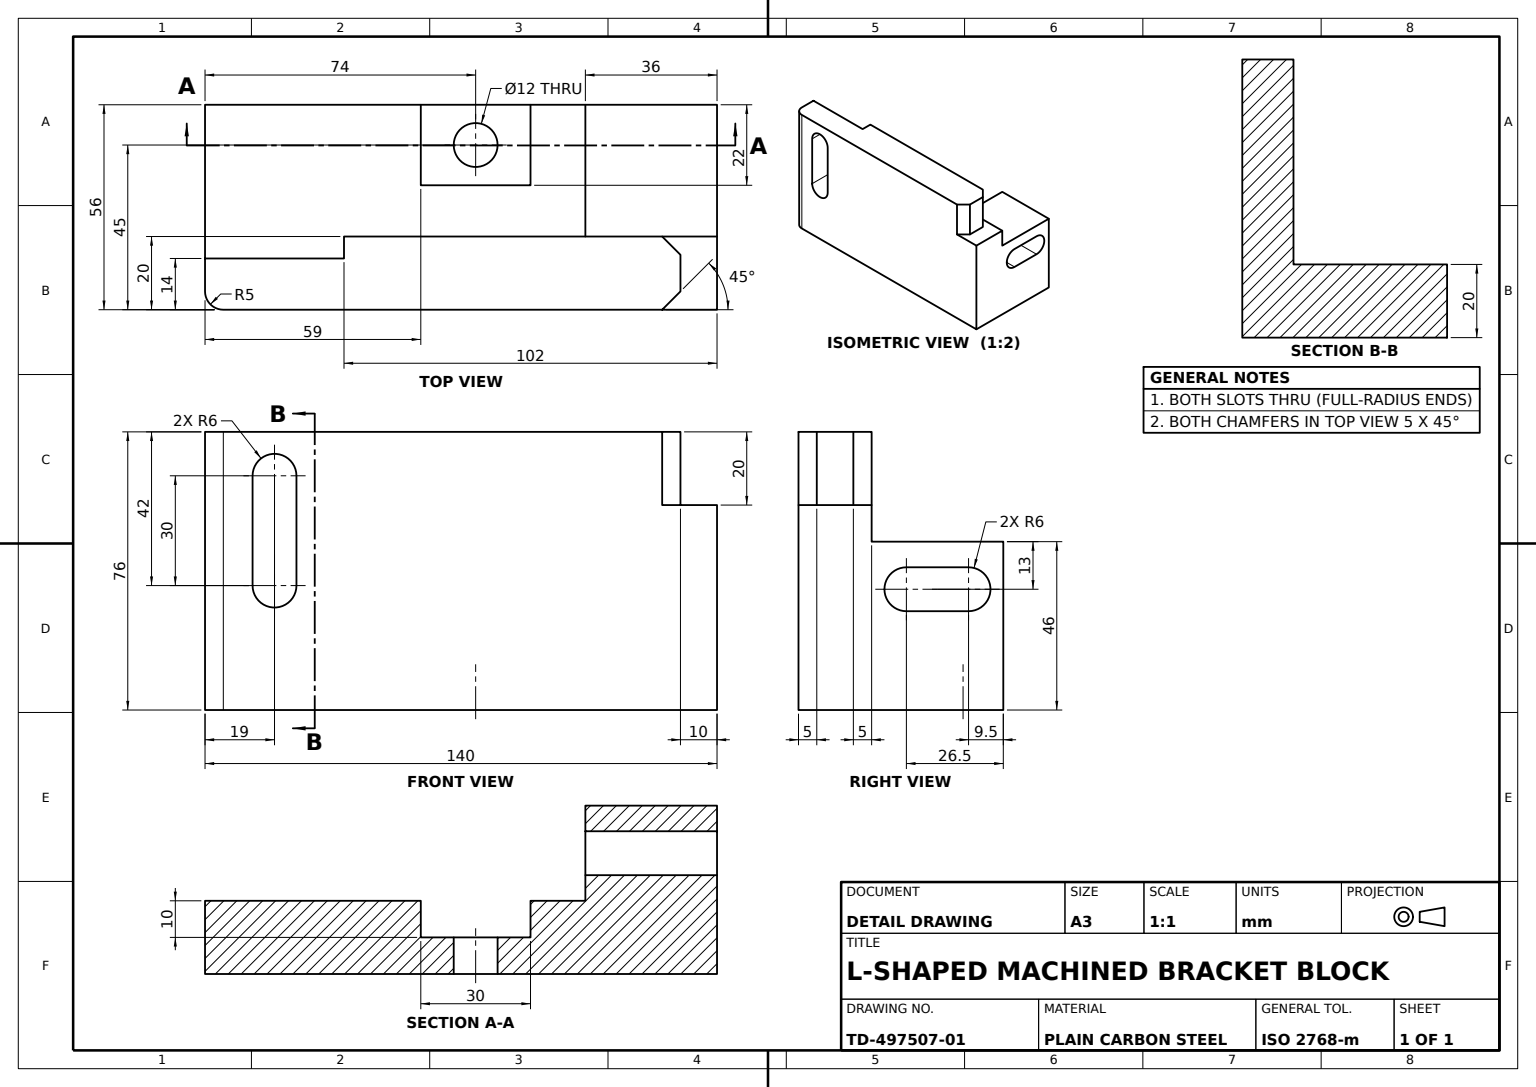
from build123d import *

# Parameters (mm, degrees)
BASE_PLATE_DEPTH            = 20
UPRIGHT_WALL_SKETCH_W       = 20
UPRIGHT_WALL_SKETCH_H       = 140
UPRIGHT_WALL_DEPTH          = 56
WALL_PROFILE_CUT_SKETCH_W   = 6
WALL_PROFILE_CUT_SKETCH_H   = 38
WALL_PROFILE_CUT_DEPTH      = 56
WALL_SLOT_DEPTH             = 56
TOP_RIDGE_SKETCH_W          = 36
TOP_RIDGE_SKETCH_H          = 46
TOP_RIDGE_DEPTH             = 36
WALL_NOTCH_SKETCH_W         = 30
WALL_NOTCH_SKETCH_H         = 10
WALL_NOTCH_DEPTH            = 22
ROUND_CUT_SKETCH_R          = 6
ROUND_CUT_DEPTH             = 65
STEP_CUT_SKETCH_W           = 10
STEP_CUT_SKETCH_H           = 20
STEP_CUT_DEPTH              = 65
STEP_CHAMFER_5MM_SIZE       = 5
BASE_EDGE_CHAMFER_5X45_SIZE = 5
CORNER_FILLET_R5_R          = 5
RIDGE_SLOT_DEPTH            = 65


with BuildPart() as part:
    # Base Plate Sketch → Base Plate (new body)
    with BuildSketch(Plane(origin=(0, 0, 0), x_dir=(1, 0, 0), z_dir=(0, 1, 0))):
        Polygon((28, 0), (28, 70), (-28, 70), (-28, -70), (28, -70), align=None)
    extrude(amount=BASE_PLATE_DEPTH)

    # Upright Wall Sketch → Upright Wall (add)
    with BuildSketch(Plane(origin=(0, 20, 0), x_dir=(1, 0, 0), z_dir=(0, 1, 0))):
        with Locations((18, 0)):
            Rectangle(UPRIGHT_WALL_SKETCH_W, UPRIGHT_WALL_SKETCH_H)
    extrude(amount=UPRIGHT_WALL_DEPTH)

    # Wall Profile Cut Sketch → Wall Profile Cut (cut)
    with BuildSketch(Plane(origin=(0, 76, 0), x_dir=(1, 0, 0), z_dir=(0, 1, 0))):
        with Locations((11, -51)):
            Rectangle(WALL_PROFILE_CUT_SKETCH_W, WALL_PROFILE_CUT_SKETCH_H)
    extrude(amount=-WALL_PROFILE_CUT_DEPTH, mode=Mode.SUBTRACT)

    # Wall Slot Sketch → Wall Slot (cut)
    with BuildSketch(Plane.ZY.offset(-14)):
        with BuildLine():
            Line((57, 64), (57, 34))
            ThreePointArc((57, 34), (51, 28), (45, 34))
            Line((45, 34), (45, 64))
            ThreePointArc((45, 64), (51, 70), (57, 64))
        make_face()
    extrude(amount=-WALL_SLOT_DEPTH, mode=Mode.SUBTRACT)

    # Top Ridge Sketch → Top Ridge (add)
    with BuildSketch(Plane.ZY.offset(28)):
        with Locations((-52, 23)):
            Rectangle(TOP_RIDGE_SKETCH_W, TOP_RIDGE_SKETCH_H)
    extrude(amount=-TOP_RIDGE_DEPTH)

    # Wall Notch Sketch → Wall Notch (cut)
    with BuildSketch(Plane.ZY.offset(28)):
        with Locations((-4, 15)):
            Rectangle(WALL_NOTCH_SKETCH_W, WALL_NOTCH_SKETCH_H)
    extrude(amount=-WALL_NOTCH_DEPTH, mode=Mode.SUBTRACT)

    # Round Cut Sketch → Round Cut (cut)
    with BuildSketch(Plane(origin=(0, 20, 0), x_dir=(1, 0, 0), z_dir=(0, 1, 0))):
        with Locations(Location((-17, 4, 0), (0, 0, 270))):
            Circle(ROUND_CUT_SKETCH_R)
    extrude(amount=-ROUND_CUT_DEPTH, mode=Mode.SUBTRACT)

    # Step Cut Sketch → Step Cut (cut)
    with BuildSketch(Plane.ZY.offset(-8)):
        with Locations((-65, 66)):
            Rectangle(STEP_CUT_SKETCH_W, STEP_CUT_SKETCH_H)
    extrude(amount=-STEP_CUT_DEPTH, mode=Mode.SUBTRACT)

    # Step Chamfer 5mm
    step_chamfer_5mm_edges = [part.edges().sort_by_distance(p)[0] for p in [
        (8, 66, -60),
    ]]
    chamfer(step_chamfer_5mm_edges, length=STEP_CHAMFER_5MM_SIZE)

    # Base Edge Chamfer 5x45
    base_edge_chamfer_5x45_edges = [part.edges().sort_by_distance(p)[0] for p in [
        (28, 66, -60),
    ]]
    chamfer(base_edge_chamfer_5x45_edges, length=BASE_EDGE_CHAMFER_5X45_SIZE)

    # Corner Fillet R5
    corner_fillet_r5_edges = [part.edges().sort_by_distance(p)[0] for p in [
        (28, 38, 70),
    ]]
    fillet(corner_fillet_r5_edges, radius=CORNER_FILLET_R5_R)

    # Ridge Slot Sketch → Ridge Slot (cut)
    with BuildSketch(Plane.XY.offset(-34)):
        with BuildLine():
            Line((-18.5, 39), (-1.5, 39))
            ThreePointArc((-1.5, 39), (4.5, 33), (-1.5, 27))
            Line((-1.5, 27), (-18.5, 27))
            ThreePointArc((-18.5, 27), (-24.5, 33), (-18.5, 39))
        make_face()
    extrude(amount=-RIDGE_SLOT_DEPTH, mode=Mode.SUBTRACT)


solid = part.part
